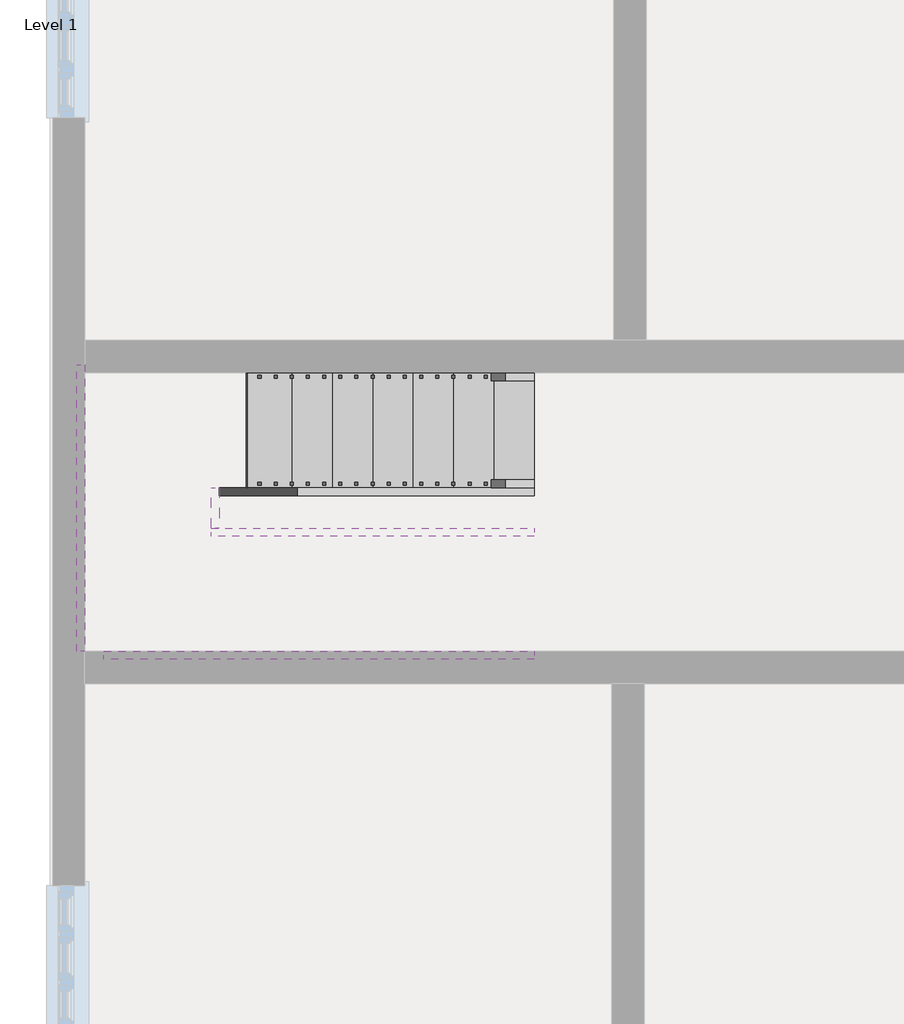
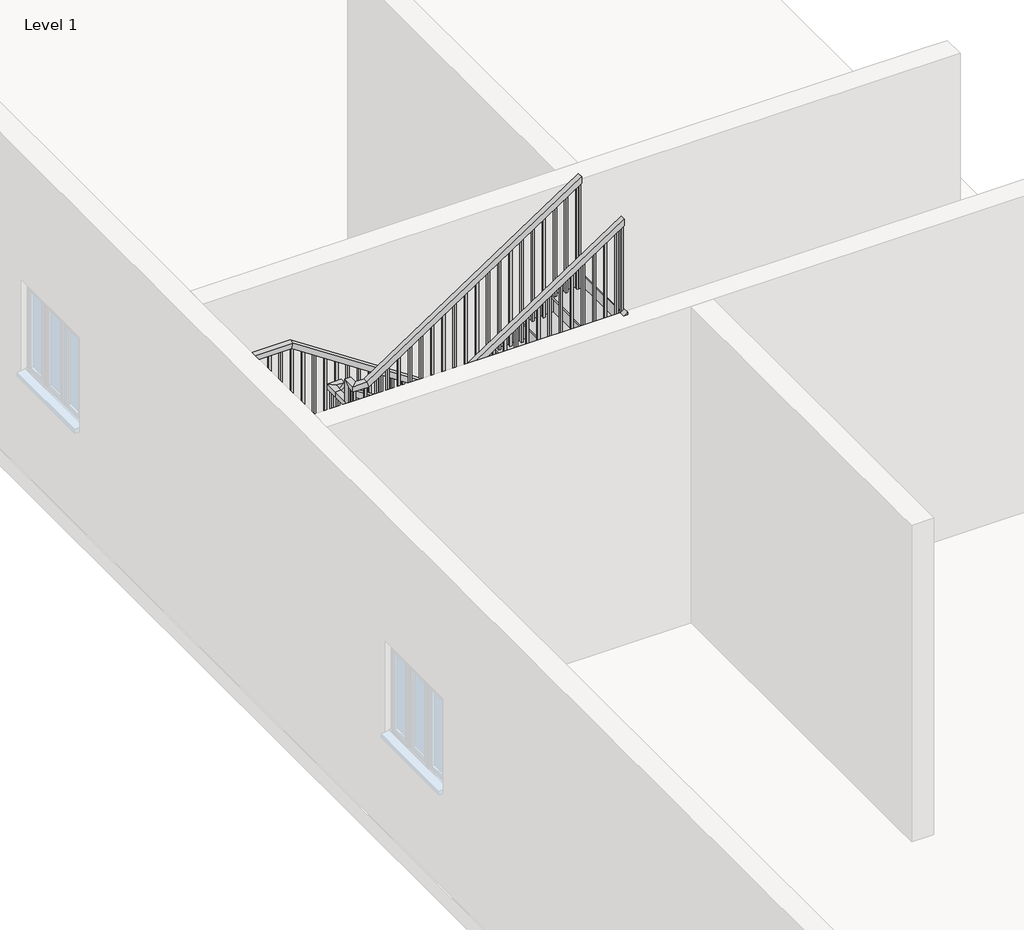
# One storey, part 2 of 2: 6 members, 2 railings, 1 stair flight.
"""IFC4 building model written with IfcOpenShell, lengths in millimetres."""

from ifc_helpers import new_model, si_unit, frame, origin, place, context, project, spatial, polyline, outline, extrude, faceted_brep, transform, mapped, element, save
from components import stair_flight_4533c53f

model = new_model("IFC4")

# Units and contexts
model_context = context("Model", 3, world=origin())
ifc_project = project(units=[si_unit("LENGTHUNIT", "METRE", prefix="MILLI")], contexts=[model_context])

# Site, building, storey
site = spatial("IfcSite", under=ifc_project)
building = spatial("IfcBuilding", under=site)
storey = spatial("IfcBuildingStorey", under=building, Name="Level 1", Elevation=0.0)

# Members
placement = place(None, origin())
element("IfcMember", 1, ObjectType="Stringer - 2\" Width", at=placement, inside=storey, context=model_context, shape_type="SweptSolid", body=[
    extrude(outline(polyline([(0.0, -2118.1728655), (217.4747739, -2118.1728655), (1527.2681072, -4099.3728655), (1161.8806735, -4099.3728655), (0.0, -2341.9063005), (0.0, -2118.1728655)])), frame((0.0, 417.8797121, 0.0), z_axis=(0.0, 1.0, 0.0), x_axis=(0.0, 0.0, 1.0)), (0.0, 0.0, 1.0), 50.8),
])
element("IfcMember", 2, ObjectType="Stringer - 2\" Width", at=placement, inside=storey, context=model_context, shape_type="SweptSolid", body=[
    extrude(outline(polyline([(-4150.1728655, 468.6797121), (-4099.3728655, 468.6797121), (-4099.3728655, 214.6797121), (-4150.1728655, 214.6797121), (-4150.1728655, 468.6797121)])), frame((0.0, 0.0, 1282.7), z_axis=(0.0, 0.0, 1.0), x_axis=(1.0, 0.0, 0.0)), (0.0, 0.0, 1.0), 304.8),
])
element("IfcMember", 3, ObjectType="Stringer - 2\" Width", at=placement, inside=storey, context=model_context, shape_type="SweptSolid", body=[
    extrude(outline(polyline([(1728.7747739, -4150.1728655), (1363.3873402, -4150.1728655), (2706.765118, -2118.1728655), (3072.1525517, -2118.1728655), (1728.7747739, -4150.1728655)])), frame((0.0, 163.8797121, 0.0), z_axis=(0.0, 1.0, 0.0), x_axis=(0.0, 0.0, 1.0)), (0.0, 0.0, 1.0), 50.8),
])
element("IfcMember", 4, ObjectType="Stringer - 2\" Width", at=placement, inside=storey, context=model_context, shape_type="SweptSolid", body=[
    extrude(outline(polyline([(0.0, -2118.1728655), (217.4747739, -2118.1728655), (1587.5, -4190.4799301), (1587.5, -4743.1668047), (0.0, -2341.9063005), (0.0, -2118.1728655)])), frame((0.0, 1192.5797121, 0.0), z_axis=(0.0, 1.0, 0.0), x_axis=(0.0, 0.0, 1.0)), (0.0, 0.0, 1.0), 50.8),
])
element("IfcMember", 5, ObjectType="Stringer - 2\" Width", at=placement, inside=storey, context=model_context, shape_type="SweptSolid", body=[
    extrude(outline(polyline([(-4994.7394105, 1243.3797121), (-4943.9394105, 1243.3797121), (-4943.9394105, -560.0202879), (-4994.7394105, -560.0202879), (-4994.7394105, 1243.3797121)])), frame((0.0, 0.0, 1282.7), z_axis=(0.0, 0.0, 1.0), x_axis=(1.0, 0.0, 0.0)), (0.0, 0.0, 1.0), 304.8),
])
element("IfcMember", 6, ObjectType="Stringer - 2\" Width", at=placement, inside=storey, context=model_context, shape_type="SweptSolid", body=[
    extrude(outline(polyline([(1282.7, -4272.2209431), (2706.765118, -2118.1728655), (3072.1525517, -2118.1728655), (1282.7, -4824.9078176), (1282.7, -4272.2209431)])), frame((0.0, -610.8202879, 0.0), z_axis=(0.0, 1.0, 0.0), x_axis=(0.0, 0.0, 1.0)), (0.0, 0.0, 1.0), 50.8),
])

# Railings
element("IfcRailing", 7, ObjectType="Handrail - Rectangular", at=placement, inside=storey, context=model_context, shape_type="SolidModel", body=[
    faceted_brep([(-2118.1728655, 1141.7797121, 1082.3222222), (-2118.1728655, 1141.7797121, 1021.4243166), (-2118.1728655, 1192.5797121, 1021.4243166), (-2118.1728655, 1192.5797121, 1082.3222222), (-4150.1728655, 1141.7797121, 2425.7), (-4165.4470084, 1141.7797121, 2374.9), (-4165.4470084, 1192.5797121, 2374.9), (-4150.1728655, 1192.5797121, 2425.7), (-4893.1394105, 1141.7797121, 2425.7), (-4893.1394105, 1141.7797121, 2374.9), (-4943.9394105, 1192.5797121, 2374.9), (-4943.9394105, 1192.5797121, 2425.7), (-4893.1394105, -509.2202879, 2425.7), (-4893.1394105, -509.2202879, 2374.9), (-4943.9394105, -560.0202879, 2374.9), (-4943.9394105, -560.0202879, 2425.7), (-4404.1728655, -509.2202879, 2425.7), (-4388.8987225, -509.2202879, 2374.9), (-4388.8987225, -560.0202879, 2374.9), (-4404.1728655, -560.0202879, 2425.7), (-2118.1728655, -509.2202879, 3937.0), (-2118.1728655, -560.0202879, 3937.0), (-2118.1728655, -560.0202879, 3876.1020944), (-2118.1728655, -509.2202879, 3876.1020944)], [[[0, 1, 2, 3]], [[1, 0, 4, 5]], [[2, 1, 5, 6]], [[3, 2, 6, 7]], [[0, 3, 7, 4]], [[5, 4, 8, 9]], [[6, 5, 9, 10]], [[7, 6, 10, 11]], [[4, 7, 11, 8]], [[9, 8, 12, 13]], [[10, 9, 13, 14]], [[11, 10, 14, 15]], [[8, 11, 15, 12]], [[13, 12, 16, 17]], [[14, 13, 17, 18]], [[15, 14, 18, 19]], [[12, 15, 19, 16]], [[20, 21, 22, 23]], [[17, 16, 20, 23]], [[18, 17, 23, 22]], [[19, 18, 22, 21]], [[16, 19, 21, 20]]]),
    extrude(outline(polyline([(3844.6057396, -2165.8144105), (3832.0115729, -2184.8644105), (2854.6777778, -2184.8644105), (2854.6777778, -2165.8144105), (3844.6057396, -2165.8144105)])), frame((0.0, -544.1452879, 0.0), z_axis=(0.0, 1.0, 0.0), x_axis=(0.0, 0.0, 1.0)), (0.0, 0.0, 1.0), 19.05),
    extrude(outline(polyline([(3777.4368507, -2267.4144105), (3764.842684, -2286.4644105), (2854.6777778, -2286.4644105), (2854.6777778, -2267.4144105), (3777.4368507, -2267.4144105)])), frame((0.0, -544.1452879, 0.0), z_axis=(0.0, 1.0, 0.0), x_axis=(0.0, 0.0, 1.0)), (0.0, 0.0, 1.0), 19.05),
    extrude(outline(polyline([(3710.2679618, -2369.0144105), (3697.6737951, -2388.0644105), (2686.7555556, -2388.0644105), (2686.7555556, -2369.0144105), (3710.2679618, -2369.0144105)])), frame((0.0, -544.1452879, 0.0), z_axis=(0.0, 1.0, 0.0), x_axis=(0.0, 0.0, 1.0)), (0.0, 0.0, 1.0), 19.05),
    extrude(outline(polyline([(3643.0990729, -2470.6144105), (3630.5049062, -2489.6644105), (2686.7555556, -2489.6644105), (2686.7555556, -2470.6144105), (3643.0990729, -2470.6144105)])), frame((0.0, -544.1452879, 0.0), z_axis=(0.0, 1.0, 0.0), x_axis=(0.0, 0.0, 1.0)), (0.0, 0.0, 1.0), 19.05),
    extrude(outline(polyline([(3576.0738572, -2572.2144105), (3563.3738572, -2591.2644105), (2686.7555556, -2591.2644105), (2686.7555556, -2572.2144105), (3576.0738572, -2572.2144105)])), frame((0.0, -544.1452879, 0.0), z_axis=(0.0, 1.0, 0.0), x_axis=(0.0, 0.0, 1.0)), (0.0, 0.0, 1.0), 19.05),
    extrude(outline(polyline([(3508.7612951, -2673.8144105), (3496.1671285, -2692.8644105), (2518.8333333, -2692.8644105), (2518.8333333, -2673.8144105), (3508.7612951, -2673.8144105)])), frame((0.0, -544.1452879, 0.0), z_axis=(0.0, 1.0, 0.0), x_axis=(0.0, 0.0, 1.0)), (0.0, 0.0, 1.0), 19.05),
    extrude(outline(polyline([(3441.5924062, -2775.4144105), (3428.9982396, -2794.4644105), (2518.8333333, -2794.4644105), (2518.8333333, -2775.4144105), (3441.5924062, -2775.4144105)])), frame((0.0, -544.1452879, 0.0), z_axis=(0.0, 1.0, 0.0), x_axis=(0.0, 0.0, 1.0)), (0.0, 0.0, 1.0), 19.05),
    extrude(outline(polyline([(3374.4235174, -2877.0144105), (3361.8293507, -2896.0644105), (2350.9111111, -2896.0644105), (2350.9111111, -2877.0144105), (3374.4235174, -2877.0144105)])), frame((0.0, -544.1452879, 0.0), z_axis=(0.0, 1.0, 0.0), x_axis=(0.0, 0.0, 1.0)), (0.0, 0.0, 1.0), 19.05),
    extrude(outline(polyline([(3307.2546285, -2978.6144105), (3294.6604618, -2997.6644105), (2350.9111111, -2997.6644105), (2350.9111111, -2978.6144105), (3307.2546285, -2978.6144105)])), frame((0.0, -544.1452879, 0.0), z_axis=(0.0, 1.0, 0.0), x_axis=(0.0, 0.0, 1.0)), (0.0, 0.0, 1.0), 19.05),
    extrude(outline(polyline([(3240.2294128, -3080.2144105), (3227.5294128, -3099.2644105), (2350.9111111, -3099.2644105), (2350.9111111, -3080.2144105), (3240.2294128, -3080.2144105)])), frame((0.0, -544.1452879, 0.0), z_axis=(0.0, 1.0, 0.0), x_axis=(0.0, 0.0, 1.0)), (0.0, 0.0, 1.0), 19.05),
    extrude(outline(polyline([(3172.9168507, -3181.8144105), (3160.322684, -3200.8644105), (2182.9888889, -3200.8644105), (2182.9888889, -3181.8144105), (3172.9168507, -3181.8144105)])), frame((0.0, -544.1452879, 0.0), z_axis=(0.0, 1.0, 0.0), x_axis=(0.0, 0.0, 1.0)), (0.0, 0.0, 1.0), 19.05),
    extrude(outline(polyline([(3105.7479618, -3283.4144105), (3093.1537951, -3302.4644105), (2182.9888889, -3302.4644105), (2182.9888889, -3283.4144105), (3105.7479618, -3283.4144105)])), frame((0.0, -544.1452879, 0.0), z_axis=(0.0, 1.0, 0.0), x_axis=(0.0, 0.0, 1.0)), (0.0, 0.0, 1.0), 19.05),
    extrude(outline(polyline([(3038.5790729, -3385.0144105), (3025.9849062, -3404.0644105), (2015.0666667, -3404.0644105), (2015.0666667, -3385.0144105), (3038.5790729, -3385.0144105)])), frame((0.0, -544.1452879, 0.0), z_axis=(0.0, 1.0, 0.0), x_axis=(0.0, 0.0, 1.0)), (0.0, 0.0, 1.0), 19.05),
    extrude(outline(polyline([(2971.410184, -3486.6144105), (2958.8160174, -3505.6644105), (2015.0666667, -3505.6644105), (2015.0666667, -3486.6144105), (2971.410184, -3486.6144105)])), frame((0.0, -544.1452879, 0.0), z_axis=(0.0, 1.0, 0.0), x_axis=(0.0, 0.0, 1.0)), (0.0, 0.0, 1.0), 19.05),
    extrude(outline(polyline([(2904.3849683, -3588.2144105), (2891.6849683, -3607.2644105), (2015.0666667, -3607.2644105), (2015.0666667, -3588.2144105), (2904.3849683, -3588.2144105)])), frame((0.0, -544.1452879, 0.0), z_axis=(0.0, 1.0, 0.0), x_axis=(0.0, 0.0, 1.0)), (0.0, 0.0, 1.0), 19.05),
    extrude(outline(polyline([(2837.0724062, -3689.8144105), (2824.4782396, -3708.8644105), (1847.1444444, -3708.8644105), (1847.1444444, -3689.8144105), (2837.0724062, -3689.8144105)])), frame((0.0, -544.1452879, 0.0), z_axis=(0.0, 1.0, 0.0), x_axis=(0.0, 0.0, 1.0)), (0.0, 0.0, 1.0), 19.05),
    extrude(outline(polyline([(2769.9035174, -3791.4144105), (2757.3093507, -3810.4644105), (1847.1444444, -3810.4644105), (1847.1444444, -3791.4144105), (2769.9035174, -3791.4144105)])), frame((0.0, -544.1452879, 0.0), z_axis=(0.0, 1.0, 0.0), x_axis=(0.0, 0.0, 1.0)), (0.0, 0.0, 1.0), 19.05),
    extrude(outline(polyline([(2702.7346285, -3893.0144105), (2690.1404618, -3912.0644105), (1679.2222222, -3912.0644105), (1679.2222222, -3893.0144105), (2702.7346285, -3893.0144105)])), frame((0.0, -544.1452879, 0.0), z_axis=(0.0, 1.0, 0.0), x_axis=(0.0, 0.0, 1.0)), (0.0, 0.0, 1.0), 19.05),
    extrude(outline(polyline([(2635.5657396, -3994.6144105), (2622.9715729, -4013.6644105), (1679.2222222, -4013.6644105), (1679.2222222, -3994.6144105), (2635.5657396, -3994.6144105)])), frame((0.0, -544.1452879, 0.0), z_axis=(0.0, 1.0, 0.0), x_axis=(0.0, 0.0, 1.0)), (0.0, 0.0, 1.0), 19.05),
    extrude(outline(polyline([(2568.5405239, -4096.2144105), (2555.8405239, -4115.2644105), (1679.2222222, -4115.2644105), (1679.2222222, -4096.2144105), (2568.5405239, -4096.2144105)])), frame((0.0, -544.1452879, 0.0), z_axis=(0.0, 1.0, 0.0), x_axis=(0.0, 0.0, 1.0)), (0.0, 0.0, 1.0), 19.05),
    extrude(outline(polyline([(2501.2279618, -4197.8144105), (2488.6337951, -4216.8644105), (1511.3, -4216.8644105), (1511.3, -4197.8144105), (2501.2279618, -4197.8144105)])), frame((0.0, -544.1452879, 0.0), z_axis=(0.0, 1.0, 0.0), x_axis=(0.0, 0.0, 1.0)), (0.0, 0.0, 1.0), 19.05),
    extrude(outline(polyline([(2434.0590729, -4299.4144105), (2421.4649062, -4318.4644105), (1511.3, -4318.4644105), (1511.3, -4299.4144105), (2434.0590729, -4299.4144105)])), frame((0.0, -544.1452879, 0.0), z_axis=(0.0, 1.0, 0.0), x_axis=(0.0, 0.0, 1.0)), (0.0, 0.0, 1.0), 19.05),
    extrude(outline(polyline([(-4420.0644105, -544.1452879), (-4420.0644105, -525.0952879), (-4401.0144105, -525.0952879), (-4401.0144105, -544.1452879), (-4420.0644105, -544.1452879)])), frame((0.0, 0.0, 1511.3), z_axis=(0.0, 0.0, 1.0), x_axis=(1.0, 0.0, 0.0)), (0.0, 0.0, 1.0), 863.6),
    extrude(outline(polyline([(-4521.6644105, -544.1452879), (-4521.6644105, -525.0952879), (-4502.6144105, -525.0952879), (-4502.6144105, -544.1452879), (-4521.6644105, -544.1452879)])), frame((0.0, 0.0, 1511.3), z_axis=(0.0, 0.0, 1.0), x_axis=(1.0, 0.0, 0.0)), (0.0, 0.0, 1.0), 863.6),
    extrude(outline(polyline([(-4623.2644105, -544.1452879), (-4623.2644105, -525.0952879), (-4604.2144105, -525.0952879), (-4604.2144105, -544.1452879), (-4623.2644105, -544.1452879)])), frame((0.0, 0.0, 1511.3), z_axis=(0.0, 0.0, 1.0), x_axis=(1.0, 0.0, 0.0)), (0.0, 0.0, 1.0), 863.6),
    extrude(outline(polyline([(-4724.8644105, -544.1452879), (-4724.8644105, -525.0952879), (-4705.8144105, -525.0952879), (-4705.8144105, -544.1452879), (-4724.8644105, -544.1452879)])), frame((0.0, 0.0, 1511.3), z_axis=(0.0, 0.0, 1.0), x_axis=(1.0, 0.0, 0.0)), (0.0, 0.0, 1.0), 863.6),
    extrude(outline(polyline([(-4826.4644105, -544.1452879), (-4826.4644105, -525.0952879), (-4807.4144105, -525.0952879), (-4807.4144105, -544.1452879), (-4826.4644105, -544.1452879)])), frame((0.0, 0.0, 1511.3), z_axis=(0.0, 0.0, 1.0), x_axis=(1.0, 0.0, 0.0)), (0.0, 0.0, 1.0), 863.6),
    extrude(outline(polyline([(-4928.0644105, -448.8952879), (-4909.0144105, -448.8952879), (-4909.0144105, -467.9452879), (-4928.0644105, -467.9452879), (-4928.0644105, -448.8952879)])), frame((0.0, 0.0, 1511.3), z_axis=(0.0, 0.0, 1.0), x_axis=(1.0, 0.0, 0.0)), (0.0, 0.0, 1.0), 863.6),
    extrude(outline(polyline([(-4928.0644105, -347.2952879), (-4909.0144105, -347.2952879), (-4909.0144105, -366.3452879), (-4928.0644105, -366.3452879), (-4928.0644105, -347.2952879)])), frame((0.0, 0.0, 1511.3), z_axis=(0.0, 0.0, 1.0), x_axis=(1.0, 0.0, 0.0)), (0.0, 0.0, 1.0), 863.6),
    extrude(outline(polyline([(-4928.0644105, -245.6952879), (-4909.0144105, -245.6952879), (-4909.0144105, -264.7452879), (-4928.0644105, -264.7452879), (-4928.0644105, -245.6952879)])), frame((0.0, 0.0, 1511.3), z_axis=(0.0, 0.0, 1.0), x_axis=(1.0, 0.0, 0.0)), (0.0, 0.0, 1.0), 863.6),
    extrude(outline(polyline([(-4928.0644105, -144.0952879), (-4909.0144105, -144.0952879), (-4909.0144105, -163.1452879), (-4928.0644105, -163.1452879), (-4928.0644105, -144.0952879)])), frame((0.0, 0.0, 1511.3), z_axis=(0.0, 0.0, 1.0), x_axis=(1.0, 0.0, 0.0)), (0.0, 0.0, 1.0), 863.6),
    extrude(outline(polyline([(-4928.0644105, -42.4952879), (-4909.0144105, -42.4952879), (-4909.0144105, -61.5452879), (-4928.0644105, -61.5452879), (-4928.0644105, -42.4952879)])), frame((0.0, 0.0, 1511.3), z_axis=(0.0, 0.0, 1.0), x_axis=(1.0, 0.0, 0.0)), (0.0, 0.0, 1.0), 863.6),
    extrude(outline(polyline([(-4928.0644105, 59.1047121), (-4909.0144105, 59.1047121), (-4909.0144105, 40.0547121), (-4928.0644105, 40.0547121), (-4928.0644105, 59.1047121)])), frame((0.0, 0.0, 1511.3), z_axis=(0.0, 0.0, 1.0), x_axis=(1.0, 0.0, 0.0)), (0.0, 0.0, 1.0), 863.6),
    extrude(outline(polyline([(-4928.0644105, 160.7047121), (-4909.0144105, 160.7047121), (-4909.0144105, 141.6547121), (-4928.0644105, 141.6547121), (-4928.0644105, 160.7047121)])), frame((0.0, 0.0, 1511.3), z_axis=(0.0, 0.0, 1.0), x_axis=(1.0, 0.0, 0.0)), (0.0, 0.0, 1.0), 863.6),
    extrude(outline(polyline([(-4928.0644105, 262.3047121), (-4909.0144105, 262.3047121), (-4909.0144105, 243.2547121), (-4928.0644105, 243.2547121), (-4928.0644105, 262.3047121)])), frame((0.0, 0.0, 1511.3), z_axis=(0.0, 0.0, 1.0), x_axis=(1.0, 0.0, 0.0)), (0.0, 0.0, 1.0), 863.6),
    extrude(outline(polyline([(-4928.0644105, 363.9047121), (-4909.0144105, 363.9047121), (-4909.0144105, 344.8547121), (-4928.0644105, 344.8547121), (-4928.0644105, 363.9047121)])), frame((0.0, 0.0, 1511.3), z_axis=(0.0, 0.0, 1.0), x_axis=(1.0, 0.0, 0.0)), (0.0, 0.0, 1.0), 863.6),
    extrude(outline(polyline([(-4928.0644105, 465.5047121), (-4909.0144105, 465.5047121), (-4909.0144105, 446.4547121), (-4928.0644105, 446.4547121), (-4928.0644105, 465.5047121)])), frame((0.0, 0.0, 1511.3), z_axis=(0.0, 0.0, 1.0), x_axis=(1.0, 0.0, 0.0)), (0.0, 0.0, 1.0), 863.6),
    extrude(outline(polyline([(-4928.0644105, 567.1047121), (-4909.0144105, 567.1047121), (-4909.0144105, 548.0547121), (-4928.0644105, 548.0547121), (-4928.0644105, 567.1047121)])), frame((0.0, 0.0, 1511.3), z_axis=(0.0, 0.0, 1.0), x_axis=(1.0, 0.0, 0.0)), (0.0, 0.0, 1.0), 863.6),
    extrude(outline(polyline([(-4928.0644105, 668.7047121), (-4909.0144105, 668.7047121), (-4909.0144105, 649.6547121), (-4928.0644105, 649.6547121), (-4928.0644105, 668.7047121)])), frame((0.0, 0.0, 1511.3), z_axis=(0.0, 0.0, 1.0), x_axis=(1.0, 0.0, 0.0)), (0.0, 0.0, 1.0), 863.6),
    extrude(outline(polyline([(-4928.0644105, 770.3047121), (-4909.0144105, 770.3047121), (-4909.0144105, 751.2547121), (-4928.0644105, 751.2547121), (-4928.0644105, 770.3047121)])), frame((0.0, 0.0, 1511.3), z_axis=(0.0, 0.0, 1.0), x_axis=(1.0, 0.0, 0.0)), (0.0, 0.0, 1.0), 863.6),
    extrude(outline(polyline([(-4928.0644105, 871.9047121), (-4909.0144105, 871.9047121), (-4909.0144105, 852.8547121), (-4928.0644105, 852.8547121), (-4928.0644105, 871.9047121)])), frame((0.0, 0.0, 1511.3), z_axis=(0.0, 0.0, 1.0), x_axis=(1.0, 0.0, 0.0)), (0.0, 0.0, 1.0), 863.6),
    extrude(outline(polyline([(-4928.0644105, 973.5047121), (-4909.0144105, 973.5047121), (-4909.0144105, 954.4547121), (-4928.0644105, 954.4547121), (-4928.0644105, 973.5047121)])), frame((0.0, 0.0, 1511.3), z_axis=(0.0, 0.0, 1.0), x_axis=(1.0, 0.0, 0.0)), (0.0, 0.0, 1.0), 863.6),
    extrude(outline(polyline([(-4928.0644105, 1075.1047121), (-4909.0144105, 1075.1047121), (-4909.0144105, 1056.0547121), (-4928.0644105, 1056.0547121), (-4928.0644105, 1075.1047121)])), frame((0.0, 0.0, 1511.3), z_axis=(0.0, 0.0, 1.0), x_axis=(1.0, 0.0, 0.0)), (0.0, 0.0, 1.0), 863.6),
    extrude(outline(polyline([(-4851.8478655, 1176.7047121), (-4851.8478655, 1157.6547121), (-4870.8978655, 1157.6547121), (-4870.8978655, 1176.7047121), (-4851.8478655, 1176.7047121)])), frame((0.0, 0.0, 1511.3), z_axis=(0.0, 0.0, 1.0), x_axis=(1.0, 0.0, 0.0)), (0.0, 0.0, 1.0), 863.6),
    extrude(outline(polyline([(-4750.2478655, 1176.7047121), (-4750.2478655, 1157.6547121), (-4769.2978655, 1157.6547121), (-4769.2978655, 1176.7047121), (-4750.2478655, 1176.7047121)])), frame((0.0, 0.0, 1511.3), z_axis=(0.0, 0.0, 1.0), x_axis=(1.0, 0.0, 0.0)), (0.0, 0.0, 1.0), 863.6),
    extrude(outline(polyline([(-4648.6478655, 1176.7047121), (-4648.6478655, 1157.6547121), (-4667.6978655, 1157.6547121), (-4667.6978655, 1176.7047121), (-4648.6478655, 1176.7047121)])), frame((0.0, 0.0, 1511.3), z_axis=(0.0, 0.0, 1.0), x_axis=(1.0, 0.0, 0.0)), (0.0, 0.0, 1.0), 863.6),
    extrude(outline(polyline([(-4547.0478655, 1176.7047121), (-4547.0478655, 1157.6547121), (-4566.0978655, 1157.6547121), (-4566.0978655, 1176.7047121), (-4547.0478655, 1176.7047121)])), frame((0.0, 0.0, 1511.3), z_axis=(0.0, 0.0, 1.0), x_axis=(1.0, 0.0, 0.0)), (0.0, 0.0, 1.0), 863.6),
    extrude(outline(polyline([(-4445.4478655, 1176.7047121), (-4445.4478655, 1157.6547121), (-4464.4978655, 1157.6547121), (-4464.4978655, 1176.7047121), (-4445.4478655, 1176.7047121)])), frame((0.0, 0.0, 1511.3), z_axis=(0.0, 0.0, 1.0), x_axis=(1.0, 0.0, 0.0)), (0.0, 0.0, 1.0), 863.6),
    extrude(outline(polyline([(-4343.8478655, 1176.7047121), (-4343.8478655, 1157.6547121), (-4362.8978655, 1157.6547121), (-4362.8978655, 1176.7047121), (-4343.8478655, 1176.7047121)])), frame((0.0, 0.0, 1511.3), z_axis=(0.0, 0.0, 1.0), x_axis=(1.0, 0.0, 0.0)), (0.0, 0.0, 1.0), 863.6),
    extrude(outline(polyline([(-4242.2478655, 1176.7047121), (-4242.2478655, 1157.6547121), (-4261.2978655, 1157.6547121), (-4261.2978655, 1176.7047121), (-4242.2478655, 1176.7047121)])), frame((0.0, 0.0, 1511.3), z_axis=(0.0, 0.0, 1.0), x_axis=(1.0, 0.0, 0.0)), (0.0, 0.0, 1.0), 863.6),
    extrude(outline(polyline([(2358.2959984, -4140.6478655), (2370.9959984, -4159.6978655), (1511.3, -4159.6978655), (1511.3, -4140.6478655), (2358.2959984, -4140.6478655)])), frame((0.0, 1157.6547121, 0.0), z_axis=(0.0, 1.0, 0.0), x_axis=(0.0, 0.0, 1.0)), (0.0, 0.0, 1.0), 19.05),
    extrude(outline(polyline([(2291.3361222, -4039.0478655), (2303.9302888, -4058.0978655), (1343.3777778, -4058.0978655), (1343.3777778, -4039.0478655), (2291.3361222, -4039.0478655)])), frame((0.0, 1157.6547121, 0.0), z_axis=(0.0, 1.0, 0.0), x_axis=(0.0, 0.0, 1.0)), (0.0, 0.0, 1.0), 19.05),
    extrude(outline(polyline([(2224.2404428, -3937.4478655), (2236.9404428, -3956.4978655), (1343.3777778, -3956.4978655), (1343.3777778, -3937.4478655), (2224.2404428, -3937.4478655)])), frame((0.0, 1157.6547121, 0.0), z_axis=(0.0, 1.0, 0.0), x_axis=(0.0, 0.0, 1.0)), (0.0, 0.0, 1.0), 19.05),
    extrude(outline(polyline([(2156.9983444, -3835.8478655), (2169.592511, -3854.8978655), (1175.4555556, -3854.8978655), (1175.4555556, -3835.8478655), (2156.9983444, -3835.8478655)])), frame((0.0, 1157.6547121, 0.0), z_axis=(0.0, 1.0, 0.0), x_axis=(0.0, 0.0, 1.0)), (0.0, 0.0, 1.0), 19.05),
    extrude(outline(polyline([(2089.8294555, -3734.2478655), (2102.4236222, -3753.2978655), (1175.4555556, -3753.2978655), (1175.4555556, -3734.2478655), (2089.8294555, -3734.2478655)])), frame((0.0, 1157.6547121, 0.0), z_axis=(0.0, 1.0, 0.0), x_axis=(0.0, 0.0, 1.0)), (0.0, 0.0, 1.0), 19.05),
    extrude(outline(polyline([(2022.451554, -3632.6478655), (2035.151554, -3651.6978655), (1175.4555556, -3651.6978655), (1175.4555556, -3632.6478655), (2022.451554, -3632.6478655)])), frame((0.0, 1157.6547121, 0.0), z_axis=(0.0, 1.0, 0.0), x_axis=(0.0, 0.0, 1.0)), (0.0, 0.0, 1.0), 19.05),
    extrude(outline(polyline([(1955.4916777, -3531.0478655), (1968.0858444, -3550.0978655), (1007.5333333, -3550.0978655), (1007.5333333, -3531.0478655), (1955.4916777, -3531.0478655)])), frame((0.0, 1157.6547121, 0.0), z_axis=(0.0, 1.0, 0.0), x_axis=(0.0, 0.0, 1.0)), (0.0, 0.0, 1.0), 19.05),
    extrude(outline(polyline([(1888.3959984, -3429.4478655), (1901.0959984, -3448.4978655), (1007.5333333, -3448.4978655), (1007.5333333, -3429.4478655), (1888.3959984, -3429.4478655)])), frame((0.0, 1157.6547121, 0.0), z_axis=(0.0, 1.0, 0.0), x_axis=(0.0, 0.0, 1.0)), (0.0, 0.0, 1.0), 19.05),
    extrude(outline(polyline([(1821.1538999, -3327.8478655), (1833.7480666, -3346.8978655), (839.6111111, -3346.8978655), (839.6111111, -3327.8478655), (1821.1538999, -3327.8478655)])), frame((0.0, 1157.6547121, 0.0), z_axis=(0.0, 1.0, 0.0), x_axis=(0.0, 0.0, 1.0)), (0.0, 0.0, 1.0), 19.05),
    extrude(outline(polyline([(1753.985011, -3226.2478655), (1766.5791777, -3245.2978655), (839.6111111, -3245.2978655), (839.6111111, -3226.2478655), (1753.985011, -3226.2478655)])), frame((0.0, 1157.6547121, 0.0), z_axis=(0.0, 1.0, 0.0), x_axis=(0.0, 0.0, 1.0)), (0.0, 0.0, 1.0), 19.05),
    extrude(outline(polyline([(1686.6071095, -3124.6478655), (1699.3071095, -3143.6978655), (839.6111111, -3143.6978655), (839.6111111, -3124.6478655), (1686.6071095, -3124.6478655)])), frame((0.0, 1157.6547121, 0.0), z_axis=(0.0, 1.0, 0.0), x_axis=(0.0, 0.0, 1.0)), (0.0, 0.0, 1.0), 19.05),
    extrude(outline(polyline([(1619.6472333, -3023.0478655), (1632.2413999, -3042.0978655), (671.6888889, -3042.0978655), (671.6888889, -3023.0478655), (1619.6472333, -3023.0478655)])), frame((0.0, 1157.6547121, 0.0), z_axis=(0.0, 1.0, 0.0), x_axis=(0.0, 0.0, 1.0)), (0.0, 0.0, 1.0), 19.05),
    extrude(outline(polyline([(1552.551554, -2921.4478655), (1565.251554, -2940.4978655), (671.6888889, -2940.4978655), (671.6888889, -2921.4478655), (1552.551554, -2921.4478655)])), frame((0.0, 1157.6547121, 0.0), z_axis=(0.0, 1.0, 0.0), x_axis=(0.0, 0.0, 1.0)), (0.0, 0.0, 1.0), 19.05),
    extrude(outline(polyline([(1485.3094555, -2819.8478655), (1497.9036222, -2838.8978655), (503.7666667, -2838.8978655), (503.7666667, -2819.8478655), (1485.3094555, -2819.8478655)])), frame((0.0, 1157.6547121, 0.0), z_axis=(0.0, 1.0, 0.0), x_axis=(0.0, 0.0, 1.0)), (0.0, 0.0, 1.0), 19.05),
    extrude(outline(polyline([(1418.1405666, -2718.2478655), (1430.7347333, -2737.2978655), (503.7666667, -2737.2978655), (503.7666667, -2718.2478655), (1418.1405666, -2718.2478655)])), frame((0.0, 1157.6547121, 0.0), z_axis=(0.0, 1.0, 0.0), x_axis=(0.0, 0.0, 1.0)), (0.0, 0.0, 1.0), 19.05),
    extrude(outline(polyline([(1350.7626651, -2616.6478655), (1363.4626651, -2635.6978655), (503.7666667, -2635.6978655), (503.7666667, -2616.6478655), (1350.7626651, -2616.6478655)])), frame((0.0, 1157.6547121, 0.0), z_axis=(0.0, 1.0, 0.0), x_axis=(0.0, 0.0, 1.0)), (0.0, 0.0, 1.0), 19.05),
    extrude(outline(polyline([(1283.8027888, -2515.0478655), (1296.3969555, -2534.0978655), (335.8444444, -2534.0978655), (335.8444444, -2515.0478655), (1283.8027888, -2515.0478655)])), frame((0.0, 1157.6547121, 0.0), z_axis=(0.0, 1.0, 0.0), x_axis=(0.0, 0.0, 1.0)), (0.0, 0.0, 1.0), 19.05),
    extrude(outline(polyline([(1216.7071095, -2413.4478655), (1229.4071095, -2432.4978655), (335.8444444, -2432.4978655), (335.8444444, -2413.4478655), (1216.7071095, -2413.4478655)])), frame((0.0, 1157.6547121, 0.0), z_axis=(0.0, 1.0, 0.0), x_axis=(0.0, 0.0, 1.0)), (0.0, 0.0, 1.0), 19.05),
    extrude(outline(polyline([(1149.465011, -2311.8478655), (1162.0591777, -2330.8978655), (167.9222222, -2330.8978655), (167.9222222, -2311.8478655), (1149.465011, -2311.8478655)])), frame((0.0, 1157.6547121, 0.0), z_axis=(0.0, 1.0, 0.0), x_axis=(0.0, 0.0, 1.0)), (0.0, 0.0, 1.0), 19.05),
    extrude(outline(polyline([(1082.2961222, -2210.2478655), (1094.8902888, -2229.2978655), (167.9222222, -2229.2978655), (167.9222222, -2210.2478655), (1082.2961222, -2210.2478655)])), frame((0.0, 1157.6547121, 0.0), z_axis=(0.0, 1.0, 0.0), x_axis=(0.0, 0.0, 1.0)), (0.0, 0.0, 1.0), 19.05),
    extrude(outline(polyline([(-4928.0644105, -525.0952879), (-4909.0144105, -525.0952879), (-4909.0144105, -544.1452879), (-4928.0644105, -544.1452879), (-4928.0644105, -525.0952879)])), frame((0.0, 0.0, 1511.3), z_axis=(0.0, 0.0, 1.0), x_axis=(1.0, 0.0, 0.0)), (0.0, 0.0, 1.0), 863.6),
    extrude(outline(polyline([(-4909.0144105, 1176.7047121), (-4909.0144105, 1157.6547121), (-4928.0644105, 1157.6547121), (-4928.0644105, 1176.7047121), (-4909.0144105, 1176.7047121)])), frame((0.0, 0.0, 1511.3), z_axis=(0.0, 0.0, 1.0), x_axis=(1.0, 0.0, 0.0)), (0.0, 0.0, 1.0), 863.6),
    extrude(outline(polyline([(3876.1020944, -2118.1728655), (3863.5079277, -2137.2228655), (2854.6777778, -2137.2228655), (2854.6777778, -2118.1728655), (3876.1020944, -2118.1728655)])), frame((0.0, -544.1452879, 0.0), z_axis=(0.0, 1.0, 0.0), x_axis=(0.0, 0.0, 1.0)), (0.0, 0.0, 1.0), 19.05),
    extrude(outline(polyline([(1021.2682206, -2118.1728655), (1033.9682206, -2137.2228655), (167.9222222, -2137.2228655), (167.9222222, -2118.1728655), (1021.2682206, -2118.1728655)])), frame((0.0, 1157.6547121, 0.0), z_axis=(0.0, 1.0, 0.0), x_axis=(0.0, 0.0, 1.0)), (0.0, 0.0, 1.0), 19.05),
])
element("IfcRailing", 8, ObjectType="Handrail - Rectangular", at=placement, inside=storey, context=model_context, shape_type="SolidModel", body=[
    faceted_brep([(-2118.1728655, 468.6797121, 1082.3222222), (-2118.1728655, 468.6797121, 1021.4243166), (-2118.1728655, 519.4797121, 1021.4243166), (-2118.1728655, 519.4797121, 1082.3222222), (-4073.9728655, 468.6797121, 2375.3233333), (-4124.7728655, 468.6797121, 2348.0098722), (-4124.7728655, 519.4797121, 2348.0098722), (-4073.9728655, 519.4797121, 2375.3233333), (-4073.9728655, 468.6797121, 2425.7), (-4124.7728655, 468.6797121, 2374.9), (-4124.7728655, 519.4797121, 2374.9), (-4073.9728655, 519.4797121, 2425.7), (-4150.1728655, 468.6797121, 2425.7), (-4150.1728655, 468.6797121, 2374.9), (-4200.9728655, 519.4797121, 2374.9), (-4200.9728655, 519.4797121, 2425.7), (-4150.1728655, 392.4797121, 2425.7), (-4150.1728655, 392.4797121, 2374.9), (-4200.9728655, 392.4797121, 2374.9), (-4200.9728655, 392.4797121, 2425.7), (-4150.1728655, 240.0797121, 2425.7), (-4150.1728655, 189.2797121, 2374.9), (-4200.9728655, 189.2797121, 2374.9), (-4200.9728655, 240.0797121, 2425.7), (-4150.1728655, 240.0797121, 2643.9988889), (-4150.1728655, 189.2797121, 2593.1988889), (-4200.9728655, 189.2797121, 2593.1988889), (-4200.9728655, 240.0797121, 2643.9988889), (-4150.1728655, 163.8797121, 2643.9988889), (-4150.1728655, 163.8797121, 2593.1988889), (-4200.9728655, 113.0797121, 2593.1988889), (-4200.9728655, 113.0797121, 2643.9988889), (-4073.9728655, 163.8797121, 2643.9988889), (-4058.6987225, 163.8797121, 2593.1988889), (-4058.6987225, 113.0797121, 2593.1988889), (-4073.9728655, 113.0797121, 2643.9988889), (-2118.1728655, 163.8797121, 3937.0), (-2118.1728655, 113.0797121, 3937.0), (-2118.1728655, 113.0797121, 3876.1020944), (-2118.1728655, 163.8797121, 3876.1020944)], [[[0, 1, 2, 3]], [[1, 0, 4, 5]], [[2, 1, 5, 6]], [[3, 2, 6, 7]], [[0, 3, 7, 4]], [[5, 4, 8, 9]], [[6, 5, 9, 10]], [[7, 6, 10, 11]], [[4, 7, 11, 8]], [[9, 8, 12, 13]], [[10, 9, 13, 14]], [[11, 10, 14, 15]], [[8, 11, 15, 12]], [[13, 12, 16, 17]], [[14, 13, 17, 18]], [[15, 14, 18, 19]], [[12, 15, 19, 16]], [[17, 16, 20, 21]], [[18, 17, 21, 22]], [[19, 18, 22, 23]], [[16, 19, 23, 20]], [[21, 20, 24, 25]], [[22, 21, 25, 26]], [[23, 22, 26, 27]], [[20, 23, 27, 24]], [[25, 24, 28, 29]], [[26, 25, 29, 30]], [[27, 26, 30, 31]], [[24, 27, 31, 28]], [[29, 28, 32, 33]], [[30, 29, 33, 34]], [[31, 30, 34, 35]], [[28, 31, 35, 32]], [[36, 37, 38, 39]], [[33, 32, 36, 39]], [[34, 33, 39, 38]], [[35, 34, 38, 37]], [[32, 35, 37, 36]]]),
    extrude(outline(polyline([(3853.0127888, -2153.0978655), (2854.6777778, -2153.0978655), (2854.6777778, -2134.0478655), (3865.6069555, -2134.0478655), (3853.0127888, -2153.0978655)])), frame((0.0, 128.9547121, 0.0), z_axis=(0.0, 1.0, 0.0), x_axis=(0.0, 0.0, 1.0)), (0.0, 0.0, 1.0), 19.05),
    extrude(outline(polyline([(3785.8438999, -2254.6978655), (2854.6777778, -2254.6978655), (2854.6777778, -2235.6478655), (3798.4380666, -2235.6478655), (3785.8438999, -2254.6978655)])), frame((0.0, 128.9547121, 0.0), z_axis=(0.0, 1.0, 0.0), x_axis=(0.0, 0.0, 1.0)), (0.0, 0.0, 1.0), 19.05),
    extrude(outline(polyline([(3718.6071095, -2356.2978655), (2854.6777778, -2356.2978655), (2854.6777778, -2337.2478655), (3731.3071095, -2337.2478655), (3718.6071095, -2356.2978655)])), frame((0.0, 128.9547121, 0.0), z_axis=(0.0, 1.0, 0.0), x_axis=(0.0, 0.0, 1.0)), (0.0, 0.0, 1.0), 19.05),
    extrude(outline(polyline([(3651.5061222, -2457.8978655), (2686.7555556, -2457.8978655), (2686.7555556, -2438.8478655), (3664.1002888, -2438.8478655), (3651.5061222, -2457.8978655)])), frame((0.0, 128.9547121, 0.0), z_axis=(0.0, 1.0, 0.0), x_axis=(0.0, 0.0, 1.0)), (0.0, 0.0, 1.0), 19.05),
    extrude(outline(polyline([(3584.3372333, -2559.4978655), (2686.7555556, -2559.4978655), (2686.7555556, -2540.4478655), (3596.9313999, -2540.4478655), (3584.3372333, -2559.4978655)])), frame((0.0, 128.9547121, 0.0), z_axis=(0.0, 1.0, 0.0), x_axis=(0.0, 0.0, 1.0)), (0.0, 0.0, 1.0), 19.05),
    extrude(outline(polyline([(3517.1683444, -2661.0978655), (2518.8333333, -2661.0978655), (2518.8333333, -2642.0478655), (3529.762511, -2642.0478655), (3517.1683444, -2661.0978655)])), frame((0.0, 128.9547121, 0.0), z_axis=(0.0, 1.0, 0.0), x_axis=(0.0, 0.0, 1.0)), (0.0, 0.0, 1.0), 19.05),
    extrude(outline(polyline([(3449.9994555, -2762.6978655), (2518.8333333, -2762.6978655), (2518.8333333, -2743.6478655), (3462.5936222, -2743.6478655), (3449.9994555, -2762.6978655)])), frame((0.0, 128.9547121, 0.0), z_axis=(0.0, 1.0, 0.0), x_axis=(0.0, 0.0, 1.0)), (0.0, 0.0, 1.0), 19.05),
    extrude(outline(polyline([(3382.7626651, -2864.2978655), (2518.8333333, -2864.2978655), (2518.8333333, -2845.2478655), (3395.4626651, -2845.2478655), (3382.7626651, -2864.2978655)])), frame((0.0, 128.9547121, 0.0), z_axis=(0.0, 1.0, 0.0), x_axis=(0.0, 0.0, 1.0)), (0.0, 0.0, 1.0), 19.05),
    extrude(outline(polyline([(3315.6616777, -2965.8978655), (2350.9111111, -2965.8978655), (2350.9111111, -2946.8478655), (3328.2558444, -2946.8478655), (3315.6616777, -2965.8978655)])), frame((0.0, 128.9547121, 0.0), z_axis=(0.0, 1.0, 0.0), x_axis=(0.0, 0.0, 1.0)), (0.0, 0.0, 1.0), 19.05),
    extrude(outline(polyline([(3248.4927888, -3067.4978655), (2350.9111111, -3067.4978655), (2350.9111111, -3048.4478655), (3261.0869555, -3048.4478655), (3248.4927888, -3067.4978655)])), frame((0.0, 128.9547121, 0.0), z_axis=(0.0, 1.0, 0.0), x_axis=(0.0, 0.0, 1.0)), (0.0, 0.0, 1.0), 19.05),
    extrude(outline(polyline([(3181.3238999, -3169.0978655), (2182.9888889, -3169.0978655), (2182.9888889, -3150.0478655), (3193.9180666, -3150.0478655), (3181.3238999, -3169.0978655)])), frame((0.0, 128.9547121, 0.0), z_axis=(0.0, 1.0, 0.0), x_axis=(0.0, 0.0, 1.0)), (0.0, 0.0, 1.0), 19.05),
    extrude(outline(polyline([(3114.155011, -3270.6978655), (2182.9888889, -3270.6978655), (2182.9888889, -3251.6478655), (3126.7491777, -3251.6478655), (3114.155011, -3270.6978655)])), frame((0.0, 128.9547121, 0.0), z_axis=(0.0, 1.0, 0.0), x_axis=(0.0, 0.0, 1.0)), (0.0, 0.0, 1.0), 19.05),
    extrude(outline(polyline([(3046.9182206, -3372.2978655), (2182.9888889, -3372.2978655), (2182.9888889, -3353.2478655), (3059.6182206, -3353.2478655), (3046.9182206, -3372.2978655)])), frame((0.0, 128.9547121, 0.0), z_axis=(0.0, 1.0, 0.0), x_axis=(0.0, 0.0, 1.0)), (0.0, 0.0, 1.0), 19.05),
    extrude(outline(polyline([(2979.8172333, -3473.8978655), (2015.0666667, -3473.8978655), (2015.0666667, -3454.8478655), (2992.4113999, -3454.8478655), (2979.8172333, -3473.8978655)])), frame((0.0, 128.9547121, 0.0), z_axis=(0.0, 1.0, 0.0), x_axis=(0.0, 0.0, 1.0)), (0.0, 0.0, 1.0), 19.05),
    extrude(outline(polyline([(2912.6483444, -3575.4978655), (2015.0666667, -3575.4978655), (2015.0666667, -3556.4478655), (2925.242511, -3556.4478655), (2912.6483444, -3575.4978655)])), frame((0.0, 128.9547121, 0.0), z_axis=(0.0, 1.0, 0.0), x_axis=(0.0, 0.0, 1.0)), (0.0, 0.0, 1.0), 19.05),
    extrude(outline(polyline([(2845.4794555, -3677.0978655), (1847.1444444, -3677.0978655), (1847.1444444, -3658.0478655), (2858.0736222, -3658.0478655), (2845.4794555, -3677.0978655)])), frame((0.0, 128.9547121, 0.0), z_axis=(0.0, 1.0, 0.0), x_axis=(0.0, 0.0, 1.0)), (0.0, 0.0, 1.0), 19.05),
    extrude(outline(polyline([(2778.3105666, -3778.6978655), (1847.1444444, -3778.6978655), (1847.1444444, -3759.6478655), (2790.9047333, -3759.6478655), (2778.3105666, -3778.6978655)])), frame((0.0, 128.9547121, 0.0), z_axis=(0.0, 1.0, 0.0), x_axis=(0.0, 0.0, 1.0)), (0.0, 0.0, 1.0), 19.05),
    extrude(outline(polyline([(2711.0737762, -3880.2978655), (1847.1444444, -3880.2978655), (1847.1444444, -3861.2478655), (2723.7737762, -3861.2478655), (2711.0737762, -3880.2978655)])), frame((0.0, 128.9547121, 0.0), z_axis=(0.0, 1.0, 0.0), x_axis=(0.0, 0.0, 1.0)), (0.0, 0.0, 1.0), 19.05),
    extrude(outline(polyline([(2643.9727888, -3981.8978655), (1679.2222222, -3981.8978655), (1679.2222222, -3962.8478655), (2656.5669555, -3962.8478655), (2643.9727888, -3981.8978655)])), frame((0.0, 128.9547121, 0.0), z_axis=(0.0, 1.0, 0.0), x_axis=(0.0, 0.0, 1.0)), (0.0, 0.0, 1.0), 19.05),
    extrude(outline(polyline([(2576.8038999, -4083.4978655), (1679.2222222, -4083.4978655), (1679.2222222, -4064.4478655), (2589.3980666, -4064.4478655), (2576.8038999, -4083.4978655)])), frame((0.0, 128.9547121, 0.0), z_axis=(0.0, 1.0, 0.0), x_axis=(0.0, 0.0, 1.0)), (0.0, 0.0, 1.0), 19.05),
    extrude(outline(polyline([(-4166.0478655, 198.8047121), (-4166.0478655, 179.7547121), (-4185.0978655, 179.7547121), (-4185.0978655, 198.8047121), (-4166.0478655, 198.8047121)])), frame((0.0, 0.0, 1511.3), z_axis=(0.0, 0.0, 1.0), x_axis=(1.0, 0.0, 0.0)), (0.0, 0.0, 1.0), 1081.8988889),
    extrude(outline(polyline([(-4166.0478655, 300.4047121), (-4166.0478655, 281.3547121), (-4185.0978655, 281.3547121), (-4185.0978655, 300.4047121), (-4166.0478655, 300.4047121)])), frame((0.0, 0.0, 1511.3), z_axis=(0.0, 0.0, 1.0), x_axis=(1.0, 0.0, 0.0)), (0.0, 0.0, 1.0), 863.6),
    extrude(outline(polyline([(-4166.0478655, 402.0047121), (-4166.0478655, 382.9547121), (-4185.0978655, 382.9547121), (-4185.0978655, 402.0047121), (-4166.0478655, 402.0047121)])), frame((0.0, 0.0, 1511.3), z_axis=(0.0, 0.0, 1.0), x_axis=(1.0, 0.0, 0.0)), (0.0, 0.0, 1.0), 863.6),
    extrude(outline(polyline([(-4140.6478655, 484.5547121), (-4159.6978655, 484.5547121), (-4159.6978655, 503.6047121), (-4140.6478655, 503.6047121), (-4140.6478655, 484.5547121)])), frame((0.0, 0.0, 1511.3), z_axis=(0.0, 0.0, 1.0), x_axis=(1.0, 0.0, 0.0)), (0.0, 0.0, 1.0), 863.6),
    extrude(outline(polyline([(2303.9302888, -4058.0978655), (1343.3777778, -4058.0978655), (1343.3777778, -4039.0478655), (2291.3361222, -4039.0478655), (2303.9302888, -4058.0978655)])), frame((0.0, 484.5547121, 0.0), z_axis=(0.0, 1.0, 0.0), x_axis=(0.0, 0.0, 1.0)), (0.0, 0.0, 1.0), 19.05),
    extrude(outline(polyline([(2236.9404428, -3956.4978655), (1343.3777778, -3956.4978655), (1343.3777778, -3937.4478655), (2224.2404428, -3937.4478655), (2236.9404428, -3956.4978655)])), frame((0.0, 484.5547121, 0.0), z_axis=(0.0, 1.0, 0.0), x_axis=(0.0, 0.0, 1.0)), (0.0, 0.0, 1.0), 19.05),
    extrude(outline(polyline([(2169.592511, -3854.8978655), (1175.4555556, -3854.8978655), (1175.4555556, -3835.8478655), (2156.9983444, -3835.8478655), (2169.592511, -3854.8978655)])), frame((0.0, 484.5547121, 0.0), z_axis=(0.0, 1.0, 0.0), x_axis=(0.0, 0.0, 1.0)), (0.0, 0.0, 1.0), 19.05),
    extrude(outline(polyline([(2102.4236222, -3753.2978655), (1175.4555556, -3753.2978655), (1175.4555556, -3734.2478655), (2089.8294555, -3734.2478655), (2102.4236222, -3753.2978655)])), frame((0.0, 484.5547121, 0.0), z_axis=(0.0, 1.0, 0.0), x_axis=(0.0, 0.0, 1.0)), (0.0, 0.0, 1.0), 19.05),
    extrude(outline(polyline([(2035.151554, -3651.6978655), (1175.4555556, -3651.6978655), (1175.4555556, -3632.6478655), (2022.451554, -3632.6478655), (2035.151554, -3651.6978655)])), frame((0.0, 484.5547121, 0.0), z_axis=(0.0, 1.0, 0.0), x_axis=(0.0, 0.0, 1.0)), (0.0, 0.0, 1.0), 19.05),
    extrude(outline(polyline([(1968.0858444, -3550.0978655), (1007.5333333, -3550.0978655), (1007.5333333, -3531.0478655), (1955.4916777, -3531.0478655), (1968.0858444, -3550.0978655)])), frame((0.0, 484.5547121, 0.0), z_axis=(0.0, 1.0, 0.0), x_axis=(0.0, 0.0, 1.0)), (0.0, 0.0, 1.0), 19.05),
    extrude(outline(polyline([(1901.0959984, -3448.4978655), (1007.5333333, -3448.4978655), (1007.5333333, -3429.4478655), (1888.3959984, -3429.4478655), (1901.0959984, -3448.4978655)])), frame((0.0, 484.5547121, 0.0), z_axis=(0.0, 1.0, 0.0), x_axis=(0.0, 0.0, 1.0)), (0.0, 0.0, 1.0), 19.05),
    extrude(outline(polyline([(1833.7480666, -3346.8978655), (839.6111111, -3346.8978655), (839.6111111, -3327.8478655), (1821.1538999, -3327.8478655), (1833.7480666, -3346.8978655)])), frame((0.0, 484.5547121, 0.0), z_axis=(0.0, 1.0, 0.0), x_axis=(0.0, 0.0, 1.0)), (0.0, 0.0, 1.0), 19.05),
    extrude(outline(polyline([(1766.5791777, -3245.2978655), (839.6111111, -3245.2978655), (839.6111111, -3226.2478655), (1753.985011, -3226.2478655), (1766.5791777, -3245.2978655)])), frame((0.0, 484.5547121, 0.0), z_axis=(0.0, 1.0, 0.0), x_axis=(0.0, 0.0, 1.0)), (0.0, 0.0, 1.0), 19.05),
    extrude(outline(polyline([(1699.3071095, -3143.6978655), (839.6111111, -3143.6978655), (839.6111111, -3124.6478655), (1686.6071095, -3124.6478655), (1699.3071095, -3143.6978655)])), frame((0.0, 484.5547121, 0.0), z_axis=(0.0, 1.0, 0.0), x_axis=(0.0, 0.0, 1.0)), (0.0, 0.0, 1.0), 19.05),
    extrude(outline(polyline([(1632.2413999, -3042.0978655), (671.6888889, -3042.0978655), (671.6888889, -3023.0478655), (1619.6472333, -3023.0478655), (1632.2413999, -3042.0978655)])), frame((0.0, 484.5547121, 0.0), z_axis=(0.0, 1.0, 0.0), x_axis=(0.0, 0.0, 1.0)), (0.0, 0.0, 1.0), 19.05),
    extrude(outline(polyline([(1565.251554, -2940.4978655), (671.6888889, -2940.4978655), (671.6888889, -2921.4478655), (1552.551554, -2921.4478655), (1565.251554, -2940.4978655)])), frame((0.0, 484.5547121, 0.0), z_axis=(0.0, 1.0, 0.0), x_axis=(0.0, 0.0, 1.0)), (0.0, 0.0, 1.0), 19.05),
    extrude(outline(polyline([(1497.9036222, -2838.8978655), (503.7666667, -2838.8978655), (503.7666667, -2819.8478655), (1485.3094555, -2819.8478655), (1497.9036222, -2838.8978655)])), frame((0.0, 484.5547121, 0.0), z_axis=(0.0, 1.0, 0.0), x_axis=(0.0, 0.0, 1.0)), (0.0, 0.0, 1.0), 19.05),
    extrude(outline(polyline([(1430.7347333, -2737.2978655), (503.7666667, -2737.2978655), (503.7666667, -2718.2478655), (1418.1405666, -2718.2478655), (1430.7347333, -2737.2978655)])), frame((0.0, 484.5547121, 0.0), z_axis=(0.0, 1.0, 0.0), x_axis=(0.0, 0.0, 1.0)), (0.0, 0.0, 1.0), 19.05),
    extrude(outline(polyline([(1363.4626651, -2635.6978655), (503.7666667, -2635.6978655), (503.7666667, -2616.6478655), (1350.7626651, -2616.6478655), (1363.4626651, -2635.6978655)])), frame((0.0, 484.5547121, 0.0), z_axis=(0.0, 1.0, 0.0), x_axis=(0.0, 0.0, 1.0)), (0.0, 0.0, 1.0), 19.05),
    extrude(outline(polyline([(1296.3969555, -2534.0978655), (335.8444444, -2534.0978655), (335.8444444, -2515.0478655), (1283.8027888, -2515.0478655), (1296.3969555, -2534.0978655)])), frame((0.0, 484.5547121, 0.0), z_axis=(0.0, 1.0, 0.0), x_axis=(0.0, 0.0, 1.0)), (0.0, 0.0, 1.0), 19.05),
    extrude(outline(polyline([(1229.4071095, -2432.4978655), (335.8444444, -2432.4978655), (335.8444444, -2413.4478655), (1216.7071095, -2413.4478655), (1229.4071095, -2432.4978655)])), frame((0.0, 484.5547121, 0.0), z_axis=(0.0, 1.0, 0.0), x_axis=(0.0, 0.0, 1.0)), (0.0, 0.0, 1.0), 19.05),
    extrude(outline(polyline([(1162.0591777, -2330.8978655), (167.9222222, -2330.8978655), (167.9222222, -2311.8478655), (1149.465011, -2311.8478655), (1162.0591777, -2330.8978655)])), frame((0.0, 484.5547121, 0.0), z_axis=(0.0, 1.0, 0.0), x_axis=(0.0, 0.0, 1.0)), (0.0, 0.0, 1.0), 19.05),
    extrude(outline(polyline([(1094.8902888, -2229.2978655), (167.9222222, -2229.2978655), (167.9222222, -2210.2478655), (1082.2961222, -2210.2478655), (1094.8902888, -2229.2978655)])), frame((0.0, 484.5547121, 0.0), z_axis=(0.0, 1.0, 0.0), x_axis=(0.0, 0.0, 1.0)), (0.0, 0.0, 1.0), 19.05),
    extrude(outline(polyline([(-4166.0478655, 148.0047121), (-4166.0478655, 128.9547121), (-4185.0978655, 128.9547121), (-4185.0978655, 148.0047121), (-4166.0478655, 148.0047121)])), frame((0.0, 0.0, 1511.3), z_axis=(0.0, 0.0, 1.0), x_axis=(1.0, 0.0, 0.0)), (0.0, 0.0, 1.0), 1081.8988889),
    extrude(outline(polyline([(-4166.0478655, 484.5547121), (-4185.0978655, 484.5547121), (-4185.0978655, 503.6047121), (-4166.0478655, 503.6047121), (-4166.0478655, 484.5547121)])), frame((0.0, 0.0, 1511.3), z_axis=(0.0, 0.0, 1.0), x_axis=(1.0, 0.0, 0.0)), (0.0, 0.0, 1.0), 863.6),
    extrude(outline(polyline([(3863.5079277, -2137.2228655), (2854.6777778, -2137.2228655), (2854.6777778, -2118.1728655), (3876.1020944, -2118.1728655), (3863.5079277, -2137.2228655)])), frame((0.0, 128.9547121, 0.0), z_axis=(0.0, 1.0, 0.0), x_axis=(0.0, 0.0, 1.0)), (0.0, 0.0, 1.0), 19.05),
    extrude(outline(polyline([(1033.9682206, -2137.2228655), (167.9222222, -2137.2228655), (167.9222222, -2118.1728655), (1021.2682206, -2118.1728655), (1033.9682206, -2137.2228655)])), frame((0.0, 484.5547121, 0.0), z_axis=(0.0, 1.0, 0.0), x_axis=(0.0, 0.0, 1.0)), (0.0, 0.0, 1.0), 19.05),
])

# Stair flight
stair_flight_shape = stair_flight_4533c53f(model_context)
element("IfcStairFlight", 9, ObjectType="2\" Tread 1\" Nosing 1/4\" Riser", at=placement, inside=storey, context=model_context, shape_type="MappedRepresentation", body=[
    mapped(stair_flight_shape, transform((0.0, 0.0, 0.0), x_axis=(1.0, 0.0, 0.0), y_axis=(0.0, 1.0, 0.0), z_axis=(0.0, 0.0, 1.0))),
])

save(model, "model.ifc")

# Revit data of these elements
# Type "Handrail - Rectangular"
#   Assembly Code = "C2010400"
#   built-in parameter 1008612 = 0.0416667 (stored number, unit not read)
#   built-in parameter 1008611 = 0.0416667 (stored number, unit not read)
#   built-in parameter 1008609 = 0.333333 (stored number, unit not read)
#   built-in parameter 1008604 = 0.166667 (stored number, unit not read)
#   built-in parameter 1008603 = 0.166667 (stored number, unit not read)
#   Railing Height = 914.4 mm
#   built-in parameter 1008630 = 2
#   built-in parameter 1008610 = 2
#   built-in parameter 1008618 = Baluster - Square : 3/4"
# Elements 1, 2, 3, 4, 5, 6 (IfcMember, "Stringer - 2\" Width")
#   Phase Created = New Construction
# Elements 7, 8 (IfcRailing, "Handrail - Rectangular")
#   Phase Created = New Construction
# Element 9 (IfcStairFlight, "2\" Tread 1\" Nosing 1/4\" Riser")
#   Phase Created = New Construction
